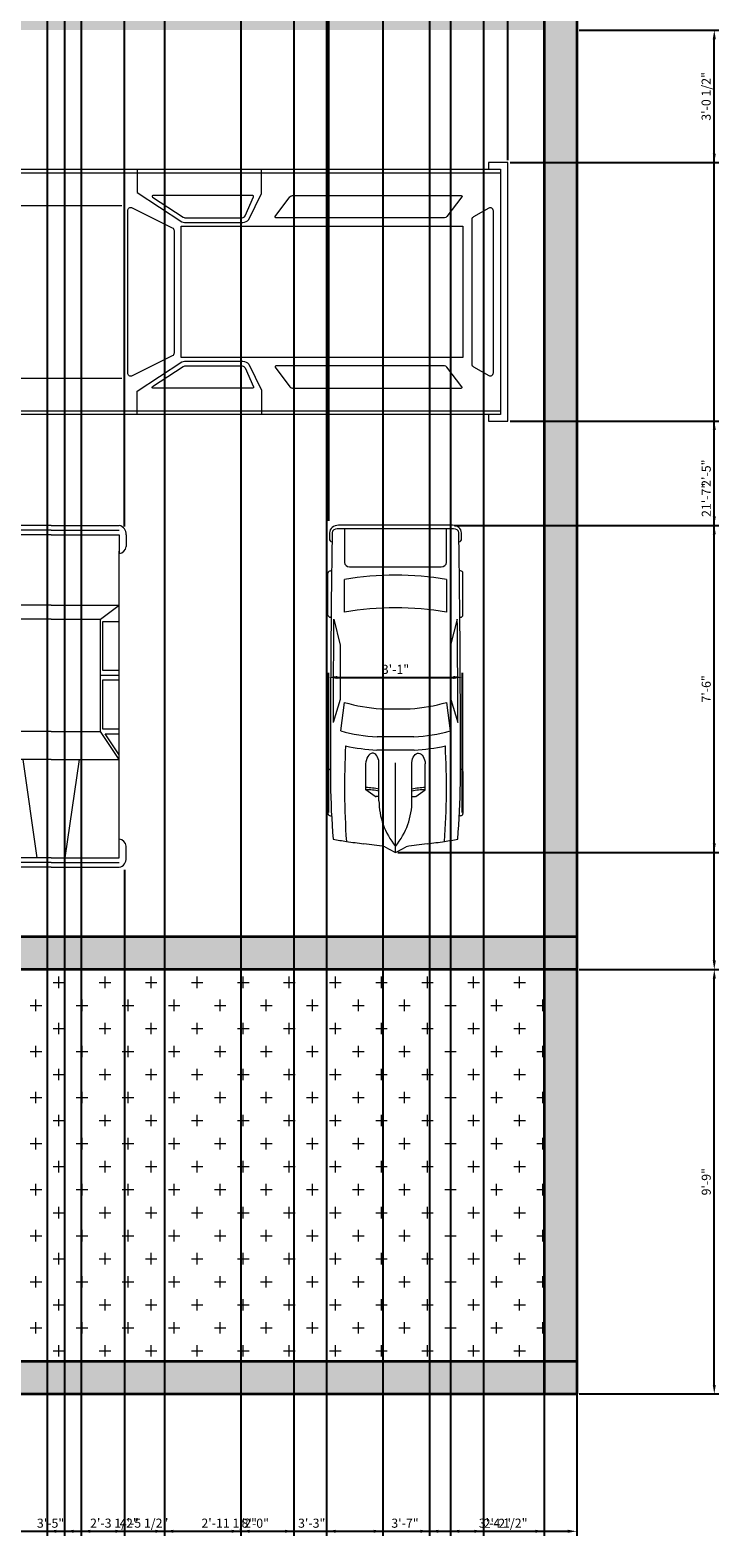
# Model space of a CAD drawing. Units: millimetres. Extents: x 2856 to 3283, y 634 to 1474.
# Tile 2 of 8: x 3092 to 3283, y 634 to 1050. Entities that reach past the tile are written whole.
import ezdxf

# ---------------------------------------------------------------- set-up
doc = ezdxf.new("R2010")
doc.units = ezdxf.units.MM
for name, color, linetype, lineweight in [('A-ANNO-DIMS', 90, 'Continuous', 18), ('A-FLOR-PATT', 50, 'Continuous', 13), ('A-WALL-PATT', 2, 'Continuous', 13), ('cars', 130, 'Continuous', 13), ('walls', 50, 'Continuous', 35)]:
    doc.layers.add(name, color=color, linetype=linetype, lineweight=lineweight)
doc.styles.get("Standard").update_dxf_attribs({"font": 'arial.ttf'})
doc.dimstyles.new('ISO-25', dxfattribs={"dimtxt": 2.5, "dimasz": 2.5, "dimexe": 1.25, "dimexo": 0.625, "dimtad": 1, "dimdec": 0, "dimlunit": 3, "dimtxsty": 'Standard', "dimcen": 2.5, "dimadec": 0, "dimazin": 0, "dimtfac": 1, "dimtdec": 0, "dimtmove": 0, "dimatfit": 3, "dimfxl": 1, "dimarcsym": 0})

# ---------------------------------------------------------------- blocks, each defined once
blk = doc.blocks.new('*U8')
for p, q in [((21.1, 37.41), (21.1, 36.83)), ((46.55, 38.89), (22.35, 38.89)), ((47.8, 37.39), (47.8, 37.41)), ((87.99, 31.87), (74.76, 35.92)), ((134.31, 35.6), (119.29, 31.78)), ((135.45, 37.07), (135.45, 37.41)), ((136.7, 38.89), (160.9, 38.89)), ((162.15, 37.41), (162.15, 36.77)), ((70.03, 31.54), (86.41, 29.35)), ((138.42, 29.35), (157.25, 29.35)), ((164.52, 26.39), (164.52, -26.39)), ((186.47, 29.35), (167.01, 29.35)), ((186.47, -33.5), (186.47, 33.5)), ((188.4, -32.76), (188.4, 32.76)), ((29.77, 9.51), (51.68, 9.51)), ((32.12, 9.51), (32.12, 11.15)), ((32.27, 11.63), (36.13, 17.17)), ((36.13, 17.17), (50.94, 17.17)), ((58.92, -10.77), (58.92, 10.77)), ((66.55, -10.53), (66.55, 10.53)), ((186.47, -10.53), (186.47, 10.53)), ((3.27, 6.13), (0.1, 0.41)), ((82.74, 8.5), (82.74, -8.5)), ((0, 0), (51.68, 0)), ((0.1, -0.41), (3.27, -6.13)), ((29.77, -9.51), (51.68, -9.51)), ((32.12, -9.51), (32.12, -11.15)), ((32.27, -11.63), (36.13, -17.17)), ((36.13, -17.17), (50.94, -17.17)), ((86.41, -29.35), (70.03, -31.54)), ((87.99, -31.87), (74.76, -35.92)), ((134.31, -35.6), (119.29, -31.78)), ((157.25, -29.35), (138.42, -29.35)), ((167.01, -29.35), (186.47, -29.35)), ((21.1, -37.41), (21.1, -36.83)), ((46.55, -38.89), (22.35, -38.89)), ((47.8, -37.39), (47.8, -37.41)), ((135.45, -37.07), (135.45, -37.41)), ((136.7, -38.89), (160.9, -38.89)), ((162.15, -37.41), (162.15, -36.77))]:
    blk.add_line(p, q)
for centre, major_axis, ratio, start_param, end_param in [((266.03, -27.52), (0, 313.31), 0.842304, 1.367076, 1.39176), ((41.19, -490.86), (0, 528.23), 0.842304, 0.00281, 0.075598), ((22.35, 37.41), (0, -1.48), 0.842304, 3.141593, 4.712389), ((64.48, -10555.62), (0, 10593.03), 0.842304, -0.013397, 0.002797), ((46.55, 37.41), (0, 1.48), 0.842304, -1.570796, 0), ((64.48, -10555.62), (0, -10591.55), 0.842304, 3.133765, 3.140441), ((136.7, 37.41), (0, -1.48), 0.842304, 3.141593, 4.712389), ((160.9, 37.41), (0, 1.48), 0.842304, -1.570796, 0), ((180.63, 35.84), (0, 2.22), 0.842304, -0.013017, 1.249894), ((64.48, -10556.36), (0, 10595.31), 0.842304, -0.013397, -0.013017), ((183.98, 33.5), (0, -2.96), 0.842304, 1.570796, 3.128196), ((183.98, 32.76), (0, -5.25), 0.842304, 1.570796, 3.128196), ((259.18, -27.52), (0, -305.3), 0.842304, 4.528606, 4.561838), ((37.47, -593.96), (0, -623.33), 0.842304, 3.096046, 3.200911), ((134.4, 5.39), (0, -89.78), 0.842304, 4.449482, 4.652344), ((135.29, 5.39), (0, 81.77), 0.842304, 1.245306, 1.50788), ((149.6, 2.8), (0, -79.58), 0.842304, 4.372215, 4.640744), ((95.79, -3666.35), (0, -3698.24), 0.842304, 3.134049, 3.144098), ((17.08, 0), (0, 147.02), 0.842304, 4.511394, 4.913384), ((35.91, 0), (0, 147.02), 0.842304, 4.511394, 4.913384), ((167.01, 26.39), (0, 2.96), 0.842304, 0, 1.570796), ((-204.49, 52.4), (0, -250.96), 0.842304, 1.385369, 1.434372), ((29.77, -46.66), (0, 56.17), 0.842304, 0, 0.590319), ((32.75, 11.15), (0, 0.74), 0.842304, 0.879714, 1.570796), ((13.04, 17.01), (0, 27.42), 0.842304, 4.435146, 4.718221), ((14.2, 17.01), (0, 27.42), 0.842304, 4.435146, 4.718221), ((50.79, 13.34), (6.34, -0.36), 0.603834, -1.395552, 1.581315), ((0.62, 0), (0, -0.74), 0.842304, 4.131459, 5.293319), ((-204.49, -52.4), (0, 250.96), 0.842304, -1.434372, -1.385369), ((29.77, 46.66), (0, 56.17), 0.842304, 2.551274, 3.141593), ((149.6, -2.8), (0, -79.58), 0.842304, -1.499151, -1.230623), ((32.75, -11.15), (0, -0.74), 0.842304, 4.712389, 5.403472), ((13.04, -17.01), (0, -27.42), 0.842304, 1.564964, 1.848039), ((14.2, -17.01), (0, -27.42), 0.842304, 1.564964, 1.848039), ((134.4, -5.39), (0, -89.78), 0.842304, -1.510751, -1.307889), ((135.29, -5.39), (0, -81.77), 0.842304, -1.50788, -1.245306), ((259.18, 27.52), (0, 305.3), 0.842304, 1.721348, 1.754579), ((266.03, 27.52), (0, 313.31), 0.842304, 1.749832, 1.774517), ((37.47, 593.96), (0, -623.33), 0.842304, -0.059319, 0.045547), ((95.79, 3666.35), (0, -3698.24), 0.842304, -0.002505, 0.007544), ((167.01, -26.39), (0, -2.96), 0.842304, 4.712389, 6.283185), ((183.98, -33.5), (0, 2.96), 0.842304, 3.15499, 4.712389), ((183.98, -32.76), (0, -5.25), 0.842304, 0.013397, 1.570796), ((41.19, 490.86), (0, -528.23), 0.842304, -0.075598, -0.00281), ((22.35, -37.41), (0, 1.48), 0.842304, 1.570796, 3.141593), ((64.48, 10555.62), (0, 10593.03), 0.842304, 3.138796, 3.15499), ((46.55, -37.41), (0, -1.48), 0.842304, 0, 1.570796), ((64.48, 10555.62), (0, -10591.55), 0.842304, 0.001152, 0.007828), ((136.7, -37.41), (0, -1.48), 0.842304, -1.570796, 0), ((160.9, -37.41), (0, 1.48), 0.842304, 3.141593, 4.712389), ((180.63, -35.84), (0, -2.22), 0.842304, -1.249894, 0.013017), ((64.48, 10556.36), (0, 10595.31), 0.842304, 3.15461, 3.15499)]:
    blk.add_ellipse(centre, major_axis=major_axis, ratio=ratio, start_param=start_param, end_param=end_param)
at = {"extrusion": (0, 0, -1)}
blk.add_ellipse((50.79, -13.34), major_axis=(6.34, 0.36), ratio=0.603834, start_param=-1.395552, end_param=1.581315, dxfattribs=at)
blk = doc.blocks.new('*U9')
for p, q in [((0.1, -0.41), (0.1, 38.35)), ((2.77, -0.41), (2.77, 38.31)), ((5.44, 42.31), (12.12, 42.31)), ((5.44, -0.41), (5.44, 38.24)), ((5.45, 38.31), (16.12, 38.31)), ((16.12, 38.31), (180.34, 38.31)), ((61.52, -0.41), (61.52, 38.31)), ((61.52, 38.31), (77.54, 27.62)), ((64.19, 38.31), (76.2, 30.29)), ((76.2, 30.29), (76.2, 38.31)), ((78.87, 38.31), (78.87, 28.96)), ((106.91, 28.96), (106.91, 38.31)), ((109.58, 27.62), (109.58, 38.31)), ((112.25, 38.31), (112.25, 28.96)), ((140.29, 28.96), (140.29, 38.31)), ((141.62, 27.62), (149.64, 38.31)), ((149.64, -0.41), (149.64, 38.31)), ((189.69, 38.31), (179.01, 38.31)), ((189.69, 42.31), (183.01, 42.31)), ((189.69, -0.41), (189.69, 38.24)), ((192.36, -0.41), (192.36, 38.31)), ((195.03, -0.41), (195.03, 38.35)), ((77.54, 27.62), (141.62, 27.62)), ((77.54, -0.41), (77.54, 27.62)), ((78.87, 28.96), (106.91, 28.96)), ((112.25, 28.96), (140.29, 28.96)), ((141.62, -0.41), (141.62, 27.62)), ((5.44, 7.6), (61.52, 15.61)), ((0.1, -0.42), (0.1, -39.18)), ((2.77, -0.41), (2.77, -39.13)), ((5.44, -0.42), (5.44, -39.07)), ((5.44, -8.42), (61.52, -16.43)), ((61.52, -0.41), (61.52, -39.13)), ((77.54, -0.41), (77.54, -28.45)), ((141.62, -0.41), (141.62, -28.45)), ((149.64, -0.41), (149.64, -39.13)), ((189.69, -0.42), (189.69, -39.07)), ((192.36, -0.41), (192.36, -39.13)), ((195.03, -0.42), (195.03, -39.18)), ((61.52, -39.13), (77.54, -28.45)), ((64.19, -39.13), (76.2, -31.12)), ((76.2, -31.12), (76.2, -39.13)), ((77.54, -28.45), (141.62, -28.45)), ((78.87, -39.13), (78.87, -29.79)), ((78.87, -29.79), (106.91, -29.79)), ((106.91, -29.79), (106.91, -39.13)), ((109.58, -28.45), (109.58, -39.13)), ((112.25, -29.79), (140.29, -29.79)), ((112.25, -39.13), (112.25, -29.79)), ((140.29, -29.79), (140.29, -39.13)), ((141.62, -28.45), (149.64, -39.13)), ((5.45, -39.13), (16.12, -39.13)), ((16.12, -39.13), (180.34, -39.13)), ((189.69, -39.13), (179.01, -39.13)), ((5.44, -43.14), (12.12, -43.14)), ((189.69, -43.14), (183.01, -43.14))]:
    blk.add_line(p, q)
for centre, radius, start, end in [((5.06, 37.26), 5.06, 85.64554, 168.0943), ((11.45, 37.64), 4.72, 8.13011, 81.86996), ((183.68, 37.64), 4.72, 98.13004, 171.8699), ((190.07, 37.26), 5.06, 11.90574, 94.35446), ((5.06, -38.09), 5.06, 191.9057, 274.3545), ((11.45, -38.46), 4.72, 278.13, 351.8699), ((183.68, -38.46), 4.72, 188.1301, 261.87), ((190.07, -38.09), 5.06, 265.6455, 348.0943)]:
    blk.add_arc(centre, radius, start, end)
blk = doc.blocks.new('*U10')
for p, q in [((1.28, 38.87), (175.66, 38.87)), ((1.28, 28.15), (52.13, 28.15)), ((1.28, -28.15), (52.13, -28.15)), ((1.28, -38.87), (175.66, -38.87))]:
    blk.add_line(p, q)
for points in [[(5.57, 40.01), (5.57, 42.18), (0, 42.18), (0, -42.18), (5.57, -42.18), (5.57, -40.01), (1.28, -40.01), (1.28, 40.01)], [(1.28, 40.01), (175.66, 40.01), (175.66, -40.01), (1.28, -40.01)], [(171.74, 40.01), (175.66, 40.01), (175.66, -40.01), (171.74, -40.01), (171.74, -42.18), (178.14, -42.18), (178.14, 42.18), (171.74, 42.18)], [(71.47, 21.48), (163.42, 21.48), (163.42, -21.48), (71.47, -21.48)]]:
    blk.add_lwpolyline(points, close=True)
for points in [[(57.15, 40.01), (57.15, 32.39), (71.72, 22.83, 0.086577), (72.56, 22.68), (91.59, 22.68, 0.227875), (93.54, 23.62), (97.72, 32.11), (97.72, 40.01)], [(57.15, -40.01), (57.15, -32.39), (71.72, -22.83, -0.086577), (72.56, -22.68), (91.59, -22.68, -0.227875), (93.54, -23.62), (97.72, -32.11), (97.72, -40.01)]]:
    blk.add_lwpolyline(points, format="xyb")
for points in [[(62.08, 30.95), (72.14, 24.35, 0.146139), (72.69, 24.18), (91.42, 24.18, 0.29766), (92.33, 24.78), (95.09, 31.05, 0.541236), (94.86, 31.41), (62.21, 31.41, 0.744989)], [(102.19, 24.58), (106.97, 31, -0.236929), (107.78, 31.41), (162.91, 31.41, -0.621576), (163.11, 31), (158.19, 24.58, -0.233368), (157.39, 24.18), (102.39, 24.18, -0.616908)], [(55.49, 27.42), (68.59, 20.89, -0.284287), (69.14, 19.99), (69.14, -19.99, -0.284287), (68.59, -20.89), (55.49, -27.42, -0.557284), (54.05, -26.53), (54.05, 26.53, -0.557284)], [(171.88, 27.31), (166.83, 24.47, 0.271143), (166.32, 23.6), (166.32, -23.6, 0.271143), (166.83, -24.47), (171.88, -27.31, 0.573387), (173.37, -26.44), (173.37, 26.44, 0.573387)], [(62.08, -30.95), (72.14, -24.35, -0.146139), (72.69, -24.18), (91.42, -24.18, -0.29766), (92.33, -24.78), (95.09, -31.05, -0.541236), (94.86, -31.41), (62.21, -31.41, -0.744989)], [(102.19, -24.58), (106.97, -31, 0.236929), (107.78, -31.41), (162.91, -31.41, 0.621576), (163.11, -31), (158.19, -24.58, 0.233368), (157.39, -24.18), (102.39, -24.18, 0.616908)]]:
    blk.add_lwpolyline(points, format="xyb", close=True)
blk = doc.blocks.new('*D28')
at = {"layer": 'A-ANNO-DIMS', "color": 0, "lineweight": -2, "transparency": 16777216}
for p, q in [((2899.17, 673.31), (2899.17, 634.81)), ((3243.17, 673.31), (3243.17, 634.81)), ((2901.67, 636.06), (3240.67, 636.06))]:
    blk.add_line(p, q, dxfattribs=at)
at = {"layer": 'A-ANNO-DIMS', "color": 0, "transparency": 16777216}
for points in [[(2901.67, 636.48), (2901.67, 635.65), (2899.17, 636.06)], [(3240.67, 636.48), (3240.67, 635.65), (3243.17, 636.06)]]:
    blk.add_solid(points, dxfattribs=at)
at = {"layer": 'Defpoints', "color": 0, "transparency": 16777216}
for p in [(2899.17, 673.94), (3243.17, 673.94), (3243.17, 636.06)]:
    blk.add_point(p, dxfattribs=at)
at = {"layer": 'A-ANNO-DIMS', "color": 0, "transparency": 16777216, "insert": (3071.17, 637.96), "char_height": 2.5, "attachment_point": 5}
blk.add_mtext('28\'-8"', dxfattribs=at)
blk = doc.blocks.new('*D30')
at = {"layer": 'A-ANNO-DIMS', "color": 0, "lineweight": -2, "transparency": 16777216}
for p, q in [((3243.8, 790.94), (3282.3, 790.94)), ((3281.05, 676.44), (3281.05, 788.44)), ((3243.8, 673.94), (3282.3, 673.94))]:
    blk.add_line(p, q, dxfattribs=at)
at = {"layer": 'A-ANNO-DIMS', "color": 0, "transparency": 16777216}
for points in [[(3280.63, 788.44), (3281.47, 788.44), (3281.05, 790.94)], [(3280.63, 676.44), (3281.47, 676.44), (3281.05, 673.94)]]:
    blk.add_solid(points, dxfattribs=at)
at = {"layer": 'Defpoints', "color": 0, "transparency": 16777216}
for p in [(3243.17, 790.94), (3281.05, 790.94), (3243.17, 673.94)]:
    blk.add_point(p, dxfattribs=at)
at = {"layer": 'A-ANNO-DIMS', "color": 0, "transparency": 16777216, "insert": (3279.15, 732.44), "char_height": 2.5, "attachment_point": 5, "rotation": 90}
blk.add_mtext('9\'-9"', dxfattribs=at)
blk = doc.blocks.new('*D31')
at = {"layer": 'A-ANNO-DIMS', "color": 0, "lineweight": -2, "transparency": 16777216}
for p, q in [((3243.8, 1049.94), (3282.3, 1049.94)), ((3281.05, 793.44), (3281.05, 1047.44)), ((3243.8, 790.94), (3282.3, 790.94))]:
    blk.add_line(p, q, dxfattribs=at)
at = {"layer": 'A-ANNO-DIMS', "color": 0, "transparency": 16777216}
for points in [[(3280.63, 1047.44), (3281.47, 1047.44), (3281.05, 1049.94)], [(3280.63, 793.44), (3281.47, 793.44), (3281.05, 790.94)]]:
    blk.add_solid(points, dxfattribs=at)
at = {"layer": 'Defpoints', "color": 0, "transparency": 16777216}
for p in [(3243.17, 1049.94), (3281.05, 1049.94), (3243.17, 790.94)]:
    blk.add_point(p, dxfattribs=at)
at = {"layer": 'A-ANNO-DIMS', "color": 0, "transparency": 16777216, "insert": (3279.17, 920.44), "char_height": 2.5, "attachment_point": 5, "rotation": 90}
blk.add_mtext('21\'-7"', dxfattribs=at)
blk = doc.blocks.new('*D33')
at = {"layer": 'A-ANNO-DIMS', "color": 0, "lineweight": -2, "transparency": 16777216}
for p, q in [((3073.7, 1014.05), (3073.7, 1470.06)), ((3076.2, 1468.81), (3221.68, 1468.81)), ((3224.18, 1014.05), (3224.18, 1470.06))]:
    blk.add_line(p, q, dxfattribs=at)
at = {"layer": 'A-ANNO-DIMS', "color": 0, "transparency": 16777216}
for points in [[(3076.2, 1469.23), (3076.2, 1468.4), (3073.7, 1468.81)], [(3221.68, 1469.23), (3221.68, 1468.4), (3224.18, 1468.81)]]:
    blk.add_solid(points, dxfattribs=at)
at = {"layer": 'Defpoints', "color": 0, "transparency": 16777216}
for p in [(3224.18, 1468.81), (3073.7, 1013.42), (3224.18, 1013.42)]:
    blk.add_point(p, dxfattribs=at)
at = {"layer": 'A-ANNO-DIMS', "color": 0, "transparency": 16777216, "insert": (3148.94, 1470.73), "char_height": 2.5, "attachment_point": 5}
blk.add_mtext('12\'-6 1/2"', dxfattribs=at)
blk = doc.blocks.new('*D36')
at = {"layer": 'A-ANNO-DIMS', "color": 0, "lineweight": -2, "transparency": 16777216}
for p, q in [((3077.68, 818.47), (3077.68, 634.81)), ((3118.46, 818.47), (3118.46, 634.81)), ((3080.18, 636.06), (3115.96, 636.06))]:
    blk.add_line(p, q, dxfattribs=at)
at = {"layer": 'A-ANNO-DIMS', "color": 0, "transparency": 16777216}
for points in [[(3080.18, 636.48), (3080.18, 635.65), (3077.68, 636.06)], [(3115.96, 636.48), (3115.96, 635.65), (3118.46, 636.06)]]:
    blk.add_solid(points, dxfattribs=at)
at = {"layer": 'Defpoints', "color": 0, "transparency": 16777216}
for p in [(3077.68, 819.09), (3118.46, 819.09), (3118.46, 636.06)]:
    blk.add_point(p, dxfattribs=at)
at = {"layer": 'A-ANNO-DIMS', "color": 0, "transparency": 16777216, "insert": (3098.07, 637.97), "char_height": 2.5, "attachment_point": 5}
blk.add_mtext('3\'-5"', dxfattribs=at)
blk = doc.blocks.new('*D37')
at = {"layer": 'A-ANNO-DIMS', "color": 0, "lineweight": -2, "transparency": 16777216}
for p, q in [((3209.46, 913.41), (3282.3, 913.41)), ((3281.05, 825.74), (3281.05, 910.91)), ((3193.78, 823.24), (3282.3, 823.24))]:
    blk.add_line(p, q, dxfattribs=at)
at = {"layer": 'A-ANNO-DIMS', "color": 0, "transparency": 16777216}
for points in [[(3280.63, 910.91), (3281.47, 910.91), (3281.05, 913.41)], [(3280.63, 825.74), (3281.47, 825.74), (3281.05, 823.24)]]:
    blk.add_solid(points, dxfattribs=at)
at = {"layer": 'Defpoints', "color": 0, "transparency": 16777216}
for p in [(3208.83, 913.41), (3281.05, 913.41), (3193.16, 823.24)]:
    blk.add_point(p, dxfattribs=at)
at = {"layer": 'A-ANNO-DIMS', "color": 0, "transparency": 16777216, "insert": (3279.15, 868.32), "char_height": 2.5, "attachment_point": 5, "rotation": 90}
blk.add_mtext('7\'-6"', dxfattribs=at)
blk = doc.blocks.new('*D38')
at = {"layer": 'A-ANNO-DIMS', "color": 0, "lineweight": -2, "transparency": 16777216}
for p, q in [((3174.66, 834.23), (3174.66, 872.73)), ((3177.16, 871.48), (3209.15, 871.48)), ((3211.65, 834.23), (3211.65, 872.73))]:
    blk.add_line(p, q, dxfattribs=at)
at = {"layer": 'A-ANNO-DIMS', "color": 0, "transparency": 16777216}
for points in [[(3177.16, 871.89), (3177.16, 871.06), (3174.66, 871.48)], [(3209.15, 871.89), (3209.15, 871.06), (3211.65, 871.48)]]:
    blk.add_solid(points, dxfattribs=at)
at = {"layer": 'Defpoints', "color": 0, "transparency": 16777216}
for p in [(3211.65, 871.48), (3174.66, 833.6), (3211.65, 833.6)]:
    blk.add_point(p, dxfattribs=at)
at = {"layer": 'A-ANNO-DIMS', "color": 0, "transparency": 16777216, "insert": (3193.16, 873.38), "char_height": 2.5, "attachment_point": 5}
blk.add_mtext('3\'-1"', dxfattribs=at)
blk = doc.blocks.new('*D40')
at = {"layer": 'A-ANNO-DIMS', "color": 0, "lineweight": -2, "transparency": 16777216}
for p, q in [((3118.44, 913.07), (3118.44, 1470.06)), ((3120.94, 1468.81), (3172.32, 1468.81)), ((3174.82, 914.65), (3174.82, 1470.06))]:
    blk.add_line(p, q, dxfattribs=at)
at = {"layer": 'A-ANNO-DIMS', "color": 0, "transparency": 16777216}
for points in [[(3120.94, 1469.23), (3120.94, 1468.4), (3118.44, 1468.81)], [(3172.32, 1469.23), (3172.32, 1468.4), (3174.82, 1468.81)]]:
    blk.add_solid(points, dxfattribs=at)
at = {"layer": 'Defpoints', "color": 0, "transparency": 16777216}
for p in [(3174.82, 1468.81), (3118.44, 912.44), (3174.82, 914.03)]:
    blk.add_point(p, dxfattribs=at)
at = {"layer": 'A-ANNO-DIMS', "color": 0, "transparency": 16777216, "insert": (3146.63, 1470.73), "char_height": 2.5, "attachment_point": 5}
blk.add_mtext('4\'-8 1/2"', dxfattribs=at)
blk = doc.blocks.new('*D41')
at = {"layer": 'A-ANNO-DIMS', "color": 0, "lineweight": -2, "transparency": 16777216}
for p, q in [((3224.8, 942.17), (3282.3, 942.17)), ((3281.05, 915.91), (3281.05, 939.67)), ((3209.46, 913.41), (3282.3, 913.41))]:
    blk.add_line(p, q, dxfattribs=at)
at = {"layer": 'A-ANNO-DIMS', "color": 0, "transparency": 16777216}
for points in [[(3280.63, 939.67), (3281.47, 939.67), (3281.05, 942.17)], [(3280.63, 915.91), (3281.47, 915.91), (3281.05, 913.41)]]:
    blk.add_solid(points, dxfattribs=at)
at = {"layer": 'Defpoints', "color": 0, "transparency": 16777216}
for p in [(3224.18, 942.17), (3281.05, 942.17), (3208.83, 913.41)]:
    blk.add_point(p, dxfattribs=at)
at = {"layer": 'A-ANNO-DIMS', "color": 0, "transparency": 16777216, "insert": (3279.15, 927.79), "char_height": 2.5, "attachment_point": 5, "rotation": 90}
blk.add_mtext('2\'-5"', dxfattribs=at)
blk = doc.blocks.new('*D42')
at = {"layer": 'A-ANNO-DIMS', "color": 0, "lineweight": -2, "transparency": 16777216}
for p, q in [((3243.8, 1049.94), (3282.3, 1049.94)), ((3281.05, 1015.92), (3281.05, 1047.44)), ((3224.8, 1013.42), (3282.3, 1013.42))]:
    blk.add_line(p, q, dxfattribs=at)
at = {"layer": 'A-ANNO-DIMS', "color": 0, "transparency": 16777216}
for points in [[(3280.63, 1047.44), (3281.47, 1047.44), (3281.05, 1049.94)], [(3280.63, 1015.92), (3281.47, 1015.92), (3281.05, 1013.42)]]:
    blk.add_solid(points, dxfattribs=at)
at = {"layer": 'Defpoints', "color": 0, "transparency": 16777216}
for p in [(3243.17, 1049.94), (3281.05, 1049.94), (3224.18, 1013.42)]:
    blk.add_point(p, dxfattribs=at)
at = {"layer": 'A-ANNO-DIMS', "color": 0, "transparency": 16777216, "insert": (3279.13, 1031.68), "char_height": 2.5, "attachment_point": 5, "rotation": 90}
blk.add_mtext('3\'-0 1/2"', dxfattribs=at)
blk = doc.blocks.new('*D55')
at = {"layer": 'A-ANNO-DIMS', "color": 0, "lineweight": -2, "transparency": 16777216}
for p, q in [((3106.52, 1060.48), (3106.52, 634.81)), ((3202.52, 1060.48), (3202.52, 634.81)), ((3109.02, 636.06), (3200.02, 636.06))]:
    blk.add_line(p, q, dxfattribs=at)
at = {"layer": 'A-ANNO-DIMS', "color": 0, "transparency": 16777216}
for points in [[(3109.02, 636.48), (3109.02, 635.65), (3106.52, 636.06)], [(3200.02, 636.48), (3200.02, 635.65), (3202.52, 636.06)]]:
    blk.add_solid(points, dxfattribs=at)
at = {"layer": 'Defpoints', "color": 0, "transparency": 16777216}
for p in [(3106.52, 1061.11), (3202.52, 1061.11), (3202.52, 636.06)]:
    blk.add_point(p, dxfattribs=at)
at = {"layer": 'A-ANNO-DIMS', "color": 0, "transparency": 16777216, "insert": (3154.52, 637.96), "char_height": 2.5, "attachment_point": 5}
blk.add_mtext('8\'-0"', dxfattribs=at)
blk = doc.blocks.new('*D57')
at = {"layer": 'A-ANNO-DIMS', "color": 0, "lineweight": -2, "transparency": 16777216}
for p, q in [((3202.52, 1060.48), (3202.52, 634.81)), ((3243.17, 1058.31), (3243.17, 634.81)), ((3205.02, 636.06), (3240.67, 636.06))]:
    blk.add_line(p, q, dxfattribs=at)
at = {"layer": 'A-ANNO-DIMS', "color": 0, "transparency": 16777216}
for points in [[(3205.02, 636.48), (3205.02, 635.65), (3202.52, 636.06)], [(3240.67, 636.48), (3240.67, 635.65), (3243.17, 636.06)]]:
    blk.add_solid(points, dxfattribs=at)
at = {"layer": 'Defpoints', "color": 0, "transparency": 16777216}
for p in [(3202.52, 1061.11), (3243.17, 1058.94), (3243.17, 636.06)]:
    blk.add_point(p, dxfattribs=at)
at = {"layer": 'A-ANNO-DIMS', "color": 0, "transparency": 16777216, "insert": (3222.85, 637.98), "char_height": 2.5, "attachment_point": 5}
blk.add_mtext('3\'-4 1/2"', dxfattribs=at)
blk = doc.blocks.new('*D62')
at = {"layer": 'A-ANNO-DIMS', "color": 0, "lineweight": -2, "transparency": 16777216}
for p, q in [((3101.93, 1287.31), (3101.93, 634.81)), ((3129.44, 1287.31), (3129.44, 634.81)), ((3104.43, 636.06), (3126.94, 636.06))]:
    blk.add_line(p, q, dxfattribs=at)
at = {"layer": 'A-ANNO-DIMS', "color": 0, "transparency": 16777216}
for points in [[(3104.43, 636.48), (3104.43, 635.65), (3101.93, 636.06)], [(3126.94, 636.48), (3126.94, 635.65), (3129.44, 636.06)]]:
    blk.add_solid(points, dxfattribs=at)
at = {"layer": 'Defpoints', "color": 0, "transparency": 16777216}
for p in [(3101.93, 1287.94), (3129.44, 1287.94), (3129.44, 636.06)]:
    blk.add_point(p, dxfattribs=at)
at = {"layer": 'A-ANNO-DIMS', "color": 0, "transparency": 16777216, "insert": (3115.68, 637.98), "char_height": 2.5, "attachment_point": 5}
blk.add_mtext('2\'-3 1/2"', dxfattribs=at)
blk = doc.blocks.new('*D71')
at = {"layer": 'A-ANNO-DIMS', "color": 0, "lineweight": -2, "transparency": 16777216}
for p, q in [((3150.5, 1421.31), (3150.5, 634.81)), ((3189.65, 1421.31), (3189.65, 634.81)), ((3153, 636.06), (3187.15, 636.06))]:
    blk.add_line(p, q, dxfattribs=at)
at = {"layer": 'A-ANNO-DIMS', "color": 0, "transparency": 16777216}
for points in [[(3153, 636.48), (3153, 635.65), (3150.5, 636.06)], [(3187.15, 636.48), (3187.15, 635.65), (3189.65, 636.06)]]:
    blk.add_solid(points, dxfattribs=at)
at = {"layer": 'Defpoints', "color": 0, "transparency": 16777216}
for p in [(3150.5, 1421.94), (3189.65, 1421.94), (3189.65, 636.06)]:
    blk.add_point(p, dxfattribs=at)
at = {"layer": 'A-ANNO-DIMS', "color": 0, "transparency": 16777216, "insert": (3170.07, 637.97), "char_height": 2.5, "attachment_point": 5}
blk.add_mtext('3\'-3"', dxfattribs=at)
blk = doc.blocks.new('*D77')
at = {"layer": 'A-ANNO-DIMS', "color": 0, "lineweight": -2, "transparency": 16777216}
for p, q in [((3097.17, 1430.31), (3097.17, 634.81)), ((3150.5, 1421.31), (3150.5, 634.81)), ((3099.67, 636.06), (3148, 636.06))]:
    blk.add_line(p, q, dxfattribs=at)
at = {"layer": 'A-ANNO-DIMS', "color": 0, "transparency": 16777216}
for points in [[(3099.67, 636.48), (3099.67, 635.65), (3097.17, 636.06)], [(3148, 636.48), (3148, 635.65), (3150.5, 636.06)]]:
    blk.add_solid(points, dxfattribs=at)
at = {"layer": 'Defpoints', "color": 0, "transparency": 16777216}
for p in [(3097.17, 1430.94), (3150.5, 1421.94), (3150.5, 636.06)]:
    blk.add_point(p, dxfattribs=at)
at = {"layer": 'A-ANNO-DIMS', "color": 0, "transparency": 16777216, "insert": (3123.84, 637.98), "char_height": 2.5, "attachment_point": 5}
blk.add_mtext('4\'-5 1/2"', dxfattribs=at)
blk = doc.blocks.new('*D80')
at = {"layer": 'A-ANNO-DIMS', "color": 0, "lineweight": -2, "transparency": 16777216}
for p, q in [((3174.17, 1239.69), (3174.17, 634.81)), ((3217.39, 1239.69), (3217.39, 634.81)), ((3176.67, 636.06), (3214.89, 636.06))]:
    blk.add_line(p, q, dxfattribs=at)
at = {"layer": 'A-ANNO-DIMS', "color": 0, "transparency": 16777216}
for points in [[(3176.67, 636.48), (3176.67, 635.65), (3174.17, 636.06)], [(3214.89, 636.48), (3214.89, 635.65), (3217.39, 636.06)]]:
    blk.add_solid(points, dxfattribs=at)
at = {"layer": 'Defpoints', "color": 0, "transparency": 16777216}
for p in [(3174.17, 1240.31), (3217.39, 1240.31), (3217.39, 636.06)]:
    blk.add_point(p, dxfattribs=at)
at = {"layer": 'A-ANNO-DIMS', "color": 0, "transparency": 16777216, "insert": (3195.78, 637.97), "char_height": 2.5, "attachment_point": 5}
blk.add_mtext('3\'-7"', dxfattribs=at)
blk = doc.blocks.new('*D88')
at = {"layer": 'A-ANNO-DIMS', "color": 0, "lineweight": -2, "transparency": 16777216}
for p, q in [((3129.44, 1287.31), (3129.44, 634.81)), ((3165.17, 1287.31), (3165.17, 634.81)), ((3131.94, 636.06), (3162.67, 636.06))]:
    blk.add_line(p, q, dxfattribs=at)
at = {"layer": 'A-ANNO-DIMS', "color": 0, "transparency": 16777216}
for points in [[(3131.94, 636.48), (3131.94, 635.65), (3129.44, 636.06)], [(3162.67, 636.48), (3162.67, 635.65), (3165.17, 636.06)]]:
    blk.add_solid(points, dxfattribs=at)
at = {"layer": 'Defpoints', "color": 0, "transparency": 16777216}
for p in [(3129.44, 1287.94), (3165.17, 1287.94), (3165.17, 636.06)]:
    blk.add_point(p, dxfattribs=at)
at = {"layer": 'A-ANNO-DIMS', "color": 0, "transparency": 16777216, "insert": (3147.31, 637.98), "char_height": 2.5, "attachment_point": 5}
blk.add_mtext('2\'-11 1/2"', dxfattribs=at)
blk = doc.blocks.new('*D92')
at = {"layer": 'A-ANNO-DIMS', "color": 0, "lineweight": -2, "transparency": 16777216}
for p, q in [((3208.3, 1343.77), (3208.3, 634.81)), ((3234.17, 1344.54), (3234.17, 634.81)), ((3210.8, 636.06), (3231.67, 636.06))]:
    blk.add_line(p, q, dxfattribs=at)
at = {"layer": 'A-ANNO-DIMS', "color": 0, "transparency": 16777216}
for points in [[(3210.8, 636.48), (3210.8, 635.65), (3208.3, 636.06)], [(3231.67, 636.48), (3231.67, 635.65), (3234.17, 636.06)]]:
    blk.add_solid(points, dxfattribs=at)
at = {"layer": 'Defpoints', "color": 0, "transparency": 16777216}
for p in [(3208.3, 1344.39), (3234.17, 1345.16), (3234.17, 636.06)]:
    blk.add_point(p, dxfattribs=at)
at = {"layer": 'A-ANNO-DIMS', "color": 0, "transparency": 16777216, "insert": (3221.24, 637.94), "char_height": 2.5, "attachment_point": 5}
blk.add_mtext('2\'-2"', dxfattribs=at)

msp = doc.modelspace()

# ---------------------------------------------------------------- hatches: boundary and pattern name
at = {"layer": 'A-FLOR-PATT'}
h = msp.add_hatch(dxfattribs=at)
h.set_pattern_fill('CROSS', color=256)
h.paths.add_polyline_path([(3234.17, 790.94), (3071.17, 790.94), (3071.17, 682.94), (3234.17, 682.94)])
at = {"layer": 'A-WALL-PATT'}
h = msp.add_hatch(color=256, dxfattribs=at)
h.dxf.hatch_style = 1
h.paths.add_polyline_path([(2908.17, 1430.94), (2899.17, 1430.94), (2899.17, 1421.94), (2908.17, 1421.94)])
h.paths.add_polyline_path([(2908.17, 1421.94), (2899.17, 1421.94), (2899.17, 1296.94), (2908.17, 1296.94)])
h.paths.add_polyline_path([(2940.27, 1430.94), (2908.17, 1430.94), (2908.17, 1421.94), (2940.27, 1421.94)])
h.paths.add_polyline_path([(3031.17, 1430.94), (2982.35, 1430.94), (2982.35, 1421.94), (3031.17, 1421.94)])
h.paths.add_polyline_path([(3150.5, 1430.94), (3097.17, 1430.94), (3097.17, 1421.94), (3150.5, 1421.94)])
h.paths.add_polyline_path([(3097.17, 1430.94), (3088.17, 1430.94), (3088.17, 1421.94), (3097.17, 1421.94)])
h.paths.add_polyline_path([(3097.17, 1421.94), (3088.17, 1421.94), (3088.17, 1337.94), (3097.17, 1337.94)])
h.paths.add_polyline_path([(3088.17, 1337.94), (3040.17, 1337.94), (3040.17, 1328.94), (3088.17, 1328.94)])
h.paths.add_polyline_path([(3097.17, 1337.94), (3088.17, 1337.94), (3088.17, 1328.94), (3097.17, 1328.94)])
h.paths.add_polyline_path([(3097.17, 1328.94), (3088.17, 1328.94), (3088.17, 1296.94), (3097.17, 1296.94)])
h.paths.add_polyline_path([(3097.17, 1296.94), (3088.17, 1296.94), (3088.17, 1287.94), (3097.17, 1287.94)])
h.paths.add_polyline_path([(3040.17, 1421.94), (3031.17, 1421.94), (3031.17, 1337.94), (3040.17, 1337.94)])
h.paths.add_polyline_path([(3040.17, 1337.94), (3031.17, 1337.94), (3031.17, 1328.94), (3040.17, 1328.94)])
h.paths.add_polyline_path([(3040.17, 1430.94), (3031.17, 1430.94), (3031.17, 1421.94), (3040.17, 1421.94)])
h.paths.add_polyline_path([(3243.17, 1421.94), (3234.17, 1421.94), (3234.17, 1385.21), (3243.17, 1385.21)])
h.paths.add_polyline_path([(3243.17, 1430.94), (3234.17, 1430.94), (3234.17, 1421.94), (3243.17, 1421.94)])
h.paths.add_polyline_path([(3234.17, 1430.94), (3189.65, 1430.94), (3189.65, 1421.94), (3234.17, 1421.94)])
h.paths.add_polyline_path([(3243.17, 1345.16), (3234.17, 1345.16), (3234.17, 1296.94), (3243.17, 1296.94)])
h.paths.add_polyline_path([(3234.17, 1296.94), (3128.45, 1296.94, -0.06768), (3129.44, 1289.59), (3129.44, 1287.94), (3234.17, 1287.94)])
h.paths.add_polyline_path([(3031.17, 1296.94), (2908.17, 1296.94), (2908.17, 1287.94), (3031.17, 1287.94)])
h.paths.add_polyline_path([(3040.17, 1296.94), (3031.17, 1296.94), (3031.17, 1287.94), (3040.17, 1287.94)])
h.paths.add_polyline_path([(2908.17, 1296.94), (2899.17, 1296.94), (2899.17, 1287.94), (2908.17, 1287.94)])
h.paths.add_polyline_path([(2908.17, 1287.94), (2899.17, 1287.94), (2899.17, 1235.12), (2908.17, 1235.12)])
h.paths.add_polyline_path([(3040.17, 1287.94), (3031.17, 1287.94), (3031.17, 1165.94), (3040.17, 1165.94)])
h.paths.add_polyline_path([(3165.17, 1165.94), (3040.17, 1165.94), (3040.17, 1156.94), (3165.17, 1156.94)])
h.paths.add_polyline_path([(3040.17, 1165.94), (3031.17, 1165.94), (3031.17, 1156.94), (3040.17, 1156.94)])
h.paths.add_polyline_path([(3040.17, 1156.94), (3031.17, 1156.94), (3031.17, 1147.75, -0.068303), (3038.59, 1148.77), (3040.17, 1148.77)])
h.paths.add_polyline_path([(3174.17, 1197.55), (3166.11, 1197.55), (3165.17, 1197.55), (3165.17, 1165.94), (3174.17, 1165.94)])
h.paths.add_polyline_path([(3174.17, 1165.94), (3165.17, 1165.94), (3165.17, 1156.94), (3174.17, 1156.94)])
h.paths.add_polyline_path([(3234.17, 1165.94), (3174.17, 1165.94), (3174.17, 1156.94), (3234.17, 1156.94)])
h.paths.add_polyline_path([(3243.17, 1165.94), (3234.17, 1165.94), (3234.17, 1156.94), (3243.17, 1156.94)])
h.paths.add_polyline_path([(3243.17, 1172.31), (3234.17, 1172.31), (3234.17, 1165.94), (3243.17, 1165.94)])
h.paths.add_polyline_path([(3243.17, 1222.94), (3234.17, 1222.94), (3234.17, 1213.94), (3243.17, 1213.94)])
h.paths.add_polyline_path([(3234.17, 1222.94), (3174.17, 1222.94), (3174.17, 1213.94), (3234.17, 1213.94)])
h.paths.add_polyline_path([(3174.17, 1222.94), (3165.17, 1222.94), (3165.17, 1213.94), (3174.17, 1213.94)])
h.paths.add_polyline_path([(3174.17, 1270.54, -0.139319), (3166.75, 1268.43), (3165.17, 1268.43), (3165.17, 1222.94), (3174.17, 1222.94)])
h.paths.add_polyline_path([(3243.17, 1243.94), (3234.17, 1243.94), (3234.17, 1222.94), (3243.17, 1222.94)])
h.paths.add_polyline_path([(3243.17, 1213.94), (3234.17, 1213.94), (3234.17, 1203.68), (3243.17, 1203.68)])
h.paths.add_polyline_path([(3174.17, 1213.94), (3165.17, 1213.94), (3165.17, 1210.62), (3166.11, 1210.62, -0.16772), (3174.17, 1207.84)])
h.paths.add_polyline_path([(3243.17, 1296.94), (3234.17, 1296.94), (3234.17, 1287.94), (3243.17, 1287.94)])
h.paths.add_polyline_path([(3243.17, 1287.94), (3234.17, 1287.94), (3234.17, 1276.76), (3243.17, 1276.76)])
h.paths.add_polyline_path([(3174.17, 1287.94), (3165.17, 1287.94), (3165.17, 1282.56), (3166.75, 1282.56), (3174.17, 1282.56)])
h.paths.add_polyline_path([(2908.17, 1190.69), (2899.17, 1190.69), (2899.17, 1116.94), (2908.17, 1116.94)])
h.paths.add_polyline_path([(2908.17, 1107.94), (2899.17, 1107.94), (2899.17, 1058.94), (2908.17, 1058.94)])
h.paths.add_polyline_path([(2908.17, 1116.94), (2899.17, 1116.94), (2899.17, 1107.94), (2908.17, 1107.94)])
h.paths.add_polyline_path([(2959.17, 1107.94), (2950.17, 1107.94), (2950.17, 1058.94), (2959.17, 1058.94)])
h.paths.add_polyline_path([(2959.17, 1116.94), (2950.17, 1116.94), (2950.17, 1107.94), (2959.17, 1107.94)])
h.paths.add_polyline_path([(2950.17, 1116.94), (2908.17, 1116.94), (2908.17, 1107.94), (2950.17, 1107.94)])
h.paths.add_polyline_path([(3031.17, 1116.94), (2959.17, 1116.94), (2959.17, 1107.94), (3031.17, 1107.94)])
h.paths.add_polyline_path([(3074.17, 1116.94), (3065.17, 1116.94), (3065.17, 1107.94), (3074.17, 1107.94)])
h.paths.add_polyline_path([(3065.17, 1116.94), (3040.17, 1116.94), (3040.17, 1107.94), (3065.17, 1107.94)])
h.paths.add_polyline_path([(3040.17, 1116.94), (3031.17, 1116.94), (3031.17, 1107.94), (3040.17, 1107.94)])
h.paths.add_polyline_path([(3040.17, 1121.26), (3038.59, 1121.26), (3031.17, 1121.26), (3031.17, 1116.94), (3040.17, 1116.94)])
h.paths.add_polyline_path([(3074.17, 1107.94), (3065.17, 1107.94), (3065.17, 1058.94), (3074.17, 1058.94)])
h.paths.add_polyline_path([(3074.17, 1058.94), (3065.17, 1058.94), (3065.17, 1049.94), (3074.17, 1049.94)])
h.paths.add_polyline_path([(3065.17, 1058.94), (2975.4, 1058.94, -0.174756), (2978.69, 1049.94), (3065.17, 1049.94)])
h.paths.add_polyline_path([(2929.83, 1051.89), (2930.25, 1058.94), (2908.17, 1058.94), (2908.17, 1049.94), (2929.71, 1049.94)])
h.paths.add_polyline_path([(2908.17, 1058.94), (2899.17, 1058.94), (2899.17, 1049.94), (2908.17, 1049.94)])
h.paths.add_polyline_path([(2950.17, 1058.94), (2942.07, 1058.94, -0.146602), (2943.93, 1051.05), (2943.86, 1049.94), (2950.17, 1049.94)])
h.paths.add_polyline_path([(2959.17, 1058.94), (2950.17, 1058.94), (2950.17, 1049.94), (2959.17, 1049.94)])
h.paths.add_polyline_path([(2964.56, 1058.94), (2959.17, 1058.94), (2959.17, 1049.94), (2964.56, 1049.94)])
h.paths.add_polyline_path([(2908.17, 1049.94), (2899.17, 1049.94), (2899.17, 799.94), (2908.17, 799.94)])
h.paths.add_polyline_path([(3234.17, 1058.94), (3074.17, 1058.94), (3074.17, 1049.94), (3234.17, 1049.94)])
h.paths.add_polyline_path([(3243.17, 1156.94), (3234.17, 1156.94), (3234.17, 1058.94), (3243.17, 1058.94)])
h.paths.add_polyline_path([(3243.17, 1058.94), (3234.17, 1058.94), (3234.17, 1049.94), (3243.17, 1049.94)])
h.paths.add_polyline_path([(3243.17, 1049.94), (3234.17, 1049.94), (3234.17, 931.7), (3234.17, 799.94), (3243.17, 799.94), (3243.17, 931.7)])
h.paths.add_polyline_path([(2908.17, 790.94), (2899.17, 790.94), (2899.17, 682.94), (2908.17, 682.94)])
h.paths.add_polyline_path([(2908.17, 799.94), (2899.17, 799.94), (2899.17, 790.94), (2908.17, 790.94)])
h.paths.add_polyline_path([(3234.17, 799.94), (2908.17, 799.94), (2908.17, 790.94), (3234.17, 790.94)])
h.paths.add_polyline_path([(3243.17, 799.94), (3234.17, 799.94), (3234.17, 790.94), (3243.17, 790.94)])
h.paths.add_polyline_path([(3243.17, 790.94), (3234.17, 790.94), (3234.17, 682.94), (3243.17, 682.94)])
h.paths.add_polyline_path([(3234.17, 682.94), (2908.17, 682.94), (2908.17, 673.94), (3234.17, 673.94)])
h.paths.add_polyline_path([(3243.17, 682.94), (3234.17, 682.94), (3234.17, 673.94), (3243.17, 673.94)])
h.paths.add_polyline_path([(2908.17, 682.94), (2899.17, 682.94), (2899.17, 673.94), (2908.17, 673.94)])

# ---------------------------------------------------------------- linework, layer by layer
at = {"layer": 'walls'}
for p, q in [((3234.17, 1287.94), (3234.17, 931.7)), ((3243.17, 1287.94), (3243.17, 931.7)), ((3234.17, 931.7), (3234.17, 790.94)), ((3243.17, 931.7), (3243.17, 790.94)), ((3243.17, 799.94), (2899.17, 799.94)), ((3243.17, 790.94), (2899.17, 790.94)), ((3234.17, 790.94), (3234.17, 673.94)), ((3243.17, 790.94), (3243.17, 673.94)), ((2899.17, 682.94), (3243.17, 682.94)), ((2899.17, 673.94), (3243.17, 673.94))]:
    msp.add_line(p, q, dxfattribs=at)

# ---------------------------------------------------------------- block references
at = {"layer": 'cars', "xscale": 0.8447207130790815, "yscale": 0.8447207130790815, "zscale": 0.8447207130790815}
msp.add_blockref('*U10', (3073.7, 977.79), dxfattribs=at)
at = {"layer": 'cars', "rotation": 90}
for name, p, xscale, yscale, zscale in [('*U9', (3098.07, 819.09), 0.4833994879051361, 0.4833994879051361, 0.4833994879051361), ('*U8', (3193.16, 823.24), 0.4786323596121468, 0.4786323596121468, 0.4786323596121468)]:
    msp.add_blockref(name, p, dxfattribs=dict(at, xscale=xscale, yscale=yscale, zscale=zscale))

# ---------------------------------------------------------------- dimensions: what is measured, and where the dimension line sits
at = {"layer": 'A-ANNO-DIMS'}
for base, p1, p2, picture, middle in [((3224.18, 1468.81), (3073.7, 1013.42), (3224.18, 1013.42), '*D33', (3148.94, 1470.73)), ((3174.82, 1468.81), (3118.44, 912.44), (3174.82, 914.03), '*D40', (3146.63, 1470.73)), ((3150.5, 636.06), (3097.17, 1430.94), (3150.5, 1421.94), '*D77', (3123.84, 637.98)), ((3189.6495, 636.0634), (3150.4985, 1421.9396), (3189.6495, 1421.9396), '*D71', (3170.074, 637.9657)), ((3234.17, 636.06), (3208.3, 1344.39), (3234.17, 1345.16), '*D92', (3221.24, 637.94)), ((3129.44, 636.06), (3101.93, 1287.94), (3129.44, 1287.94), '*D62', (3115.68, 637.98)), ((3165.17, 636.06), (3129.44, 1287.94), (3165.17, 1287.94), '*D88', (3147.31, 637.98)), ((3217.39, 636.06), (3174.17, 1240.31), (3217.39, 1240.31), '*D80', (3195.78, 637.97)), ((3202.52, 636.06), (3106.52, 1061.11), (3202.52, 1061.11), '*D55', (3154.52, 637.96)), ((3243.1743, 636.0634), (3202.518, 1061.1095), (3243.1743, 1058.9396), '*D57', (3222.8462, 637.9819)), ((3211.65, 871.48), (3174.66, 833.6), (3211.65, 833.6), '*D38', (3193.16, 873.38)), ((3118.46, 636.06), (3077.68, 819.09), (3118.46, 819.09), '*D36', (3098.07, 637.97)), ((3243.17, 636.06), (2899.17, 673.94), (3243.17, 673.94), '*D28', (3071.17, 637.96))]:
    dim = msp.add_linear_dim(base=base, p1=p1, p2=p2, dimstyle='ISO-25', override={"dimdec": 1, "dimlfac": 1, "dimrnd": 0, "dimzin": 1, "dimdsep": 46, "dimlunit": 4, "dimfrac": 2}, dxfattribs=at)
    dim.commit()
    dim.dimension.update_dxf_attribs({"geometry": picture, "text_midpoint": middle})
for base, p1, p2, picture, middle in [((3281.05, 1049.94), (3224.18, 1013.42), (3243.17, 1049.94), '*D42', (3279.13, 1031.68)), ((3281.05, 1049.94), (3243.17, 790.94), (3243.17, 1049.94), '*D31', (3279.17, 920.44)), ((3281.05, 942.17), (3208.83, 913.41), (3224.18, 942.17), '*D41', (3279.15, 927.79)), ((3281.05, 913.41), (3193.16, 823.24), (3208.83, 913.41), '*D37', (3279.15, 868.32)), ((3281.05, 790.94), (3243.17, 673.94), (3243.17, 790.94), '*D30', (3279.15, 732.44))]:
    dim = msp.add_linear_dim(base=base, p1=p1, p2=p2, angle=90, dimstyle='ISO-25', override={"dimdec": 1, "dimlfac": 1, "dimrnd": 0, "dimzin": 1, "dimdsep": 46, "dimlunit": 4, "dimfrac": 2}, dxfattribs=at)
    dim.commit()
    dim.dimension.update_dxf_attribs({"geometry": picture, "text_midpoint": middle})

doc.saveas('drawing.dxf')
